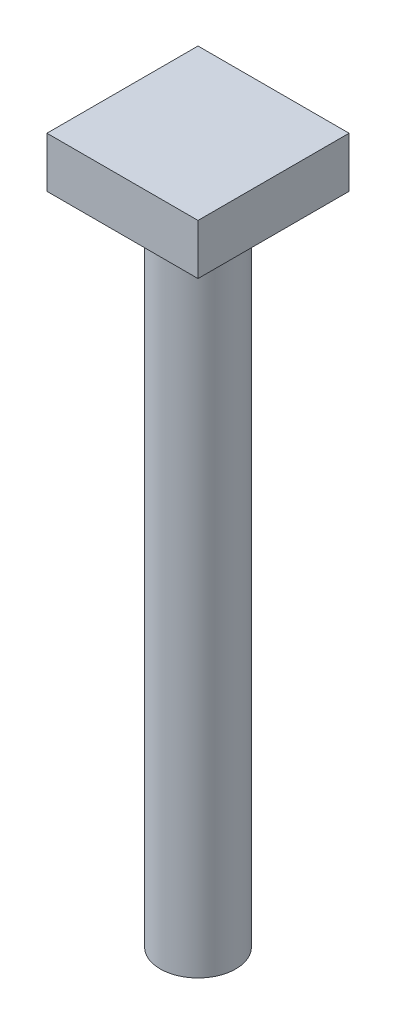
from build123d import *

# Parameters (mm, degrees)
HEAD_PROFILE_24X24_W      = 24
HEAD_PROFILE_24X24_H      = 24
SQUARE_HEAD_24X24X8_DEPTH = 8
SHANK_PROFILE_12_R        = 6
SHANK_12X104_DEPTH        = 104


with BuildPart() as part:
    # Head Profile 24x24 → Square Head 24x24x8 (new body)
    with BuildSketch(Plane(origin=(0, 0, 0), x_dir=(1, 0, 0), z_dir=(0, 1, 0))):
        Rectangle(HEAD_PROFILE_24X24_W, HEAD_PROFILE_24X24_H)
    extrude(amount=SQUARE_HEAD_24X24X8_DEPTH)

    # Shank Profile Ø12 → Shank Ø12x104 (add)
    with BuildSketch(Plane.XZ):
        with Locations(Location((0, 0, 0), (0, 0, 90))):
            Circle(SHANK_PROFILE_12_R)
    extrude(amount=SHANK_12X104_DEPTH)


solid = part.part
